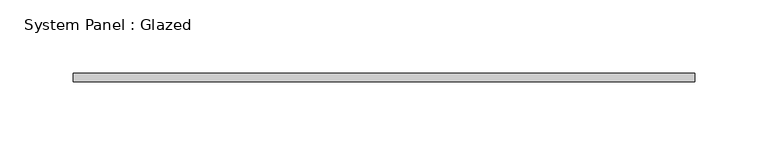
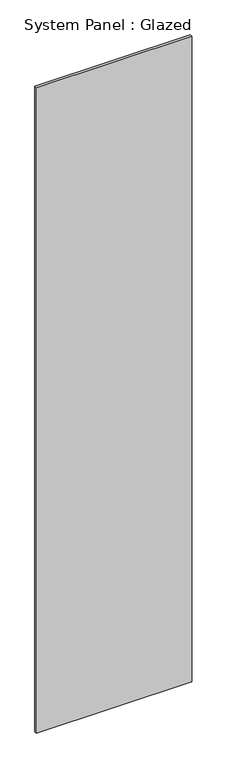
"""IFC4 building model written with IfcOpenShell, lengths in millimetres: plate geometry, System Panel : Glazed."""

from ifc_helpers import new_model, si_unit, origin, origin_with_axes, place, context, project, spatial, polyline, outline, extrude, source, transform, mapped, element, save


def system_panel_glazed_03cdf4a0(model_context):
    return source(origin(), model_context, "Body", "SweptSolid", [
        extrude(outline(polyline([(212.5, 34.0), (-212.5, 34.0), (-212.5, 40.0), (212.5, 40.0), (212.5, 34.0)])), origin_with_axes(), (0.0, 0.0, 1.0), 1865.4113705),
    ])


if __name__ == "__main__":
    model = new_model("IFC4")
    model_context = context("Model", 3, world=origin())
    ifc_project = project(units=[si_unit("LENGTHUNIT", "METRE", prefix="MILLI")], contexts=[model_context])
    site = spatial("IfcSite", under=ifc_project)
    building = spatial("IfcBuilding", under=site)
    placement = place(None, origin())
    system_panel_glazed_shape = system_panel_glazed_03cdf4a0(model_context)
    element("IfcPlate", 1, ObjectType="System Panel : Glazed", at=placement, inside=building, context=model_context, shape_type="MappedRepresentation", body=[
        mapped(system_panel_glazed_shape, transform((0.0, 0.0, 0.0), x_axis=(1.0, 0.0, 0.0), y_axis=(0.0, 1.0, 0.0), z_axis=(0.0, 0.0, 1.0))),
    ])
    save(model, "model.ifc")

# Revit data of these elements
# Type "System Panel : Glazed"
#   Construction Type Id = "GSP4R"
#   Analytic Construction = "1/8 in Pilkington single glazing"
#   Visual Light Transmittance = 0.9
#   Solar Heat Gain Coefficient = 0.86
#   Heat Transfer Coefficient (U) = 6.7069 W/(m²·K)
#   Define Thermal Properties by = 1
# Element 1 (IfcPlate, "System Panel : Glazed")
#   Materials on its faces: "Default New Material(6)"
# Materials
#   "Default New Material(6)": class "Generic", colour RGB 191 25 25, transparency 0.9, Cost = 0
